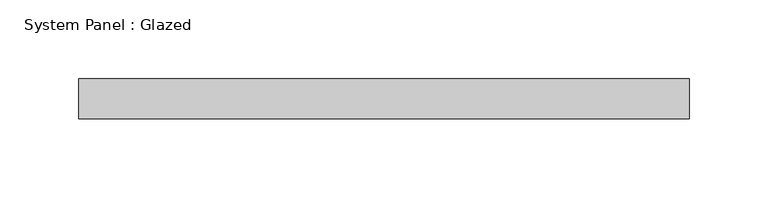
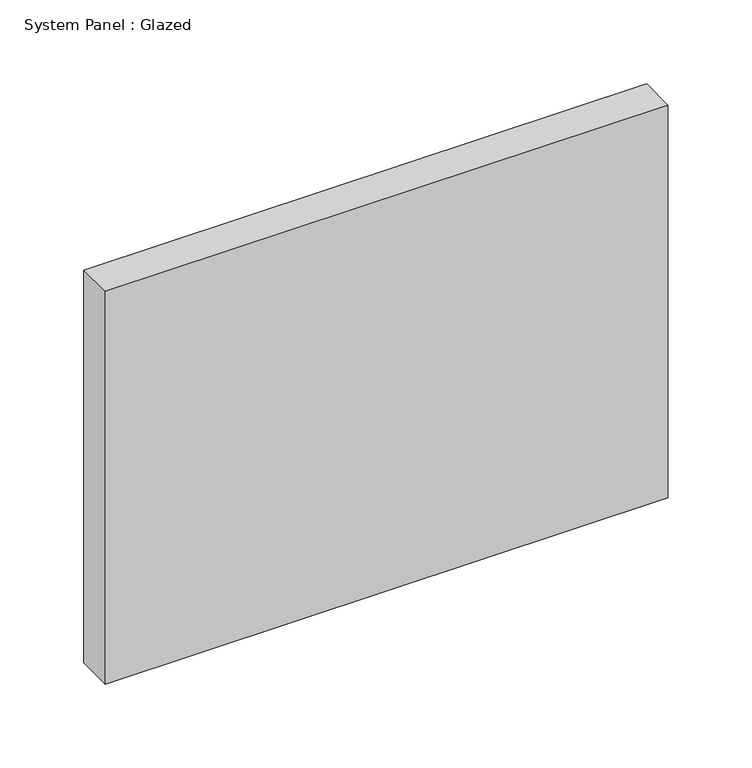
"""IFC4 building model written with IfcOpenShell, lengths in millimetres: plate geometry, System Panel : Glazed."""

from ifc_helpers import new_model, si_unit, origin, origin_with_axes, place, context, project, spatial, polyline, outline, extrude, source, transform, mapped, element, save


def system_panel_glazed_7704e2d2(model_context):
    return source(origin(), model_context, "Body", "SweptSolid", [
        extrude(outline(polyline([(193.675, 19.05), (-193.675, 19.05), (-193.675, 44.45), (193.675, 44.45), (193.675, 19.05)])), origin_with_axes(), (0.0, 0.0, 1.0), 285.75),
    ])


if __name__ == "__main__":
    model = new_model("IFC4")
    model_context = context("Model", 3, world=origin())
    ifc_project = project(units=[si_unit("LENGTHUNIT", "METRE", prefix="MILLI")], contexts=[model_context])
    site = spatial("IfcSite", under=ifc_project)
    building = spatial("IfcBuilding", under=site)
    placement = place(None, origin())
    system_panel_glazed_shape = system_panel_glazed_7704e2d2(model_context)
    element("IfcPlate", 1, ObjectType="System Panel : Glazed", at=placement, inside=building, context=model_context, shape_type="MappedRepresentation", body=[
        mapped(system_panel_glazed_shape, transform((0.0, 0.0, 0.0), x_axis=(1.0, 0.0, 0.0), y_axis=(0.0, 1.0, 0.0), z_axis=(0.0, 0.0, 1.0))),
    ])
    save(model, "model.ifc")

# Revit data of these elements
# Type "System Panel : Glazed"
#   Construction Type Id = "GSP4R"
#   Analytic Construction = "1/8 in Pilkington single glazing"
#   Visual Light Transmittance = 0.9
#   Solar Heat Gain Coefficient = 0.86
#   Heat Transfer Coefficient (U) = 1.18115 BTU/(h·ft²·°F)
#   Define Thermal Properties by = 1
# Element 1 (IfcPlate, "System Panel : Glazed")
#   Materials on its faces: "Glass"
# Materials
#   "Glass": class "Glass", colour RGB 0 128 192, transparency 0.75, Description = "Soda Lime Glass", Cost = 0
